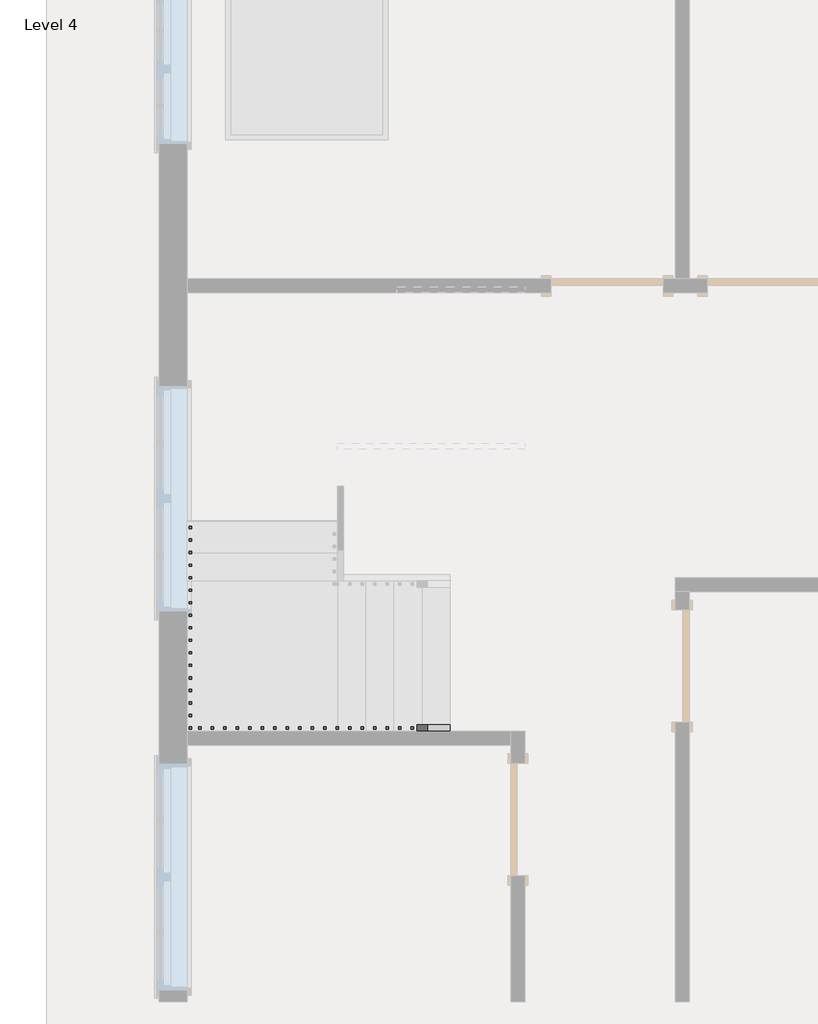
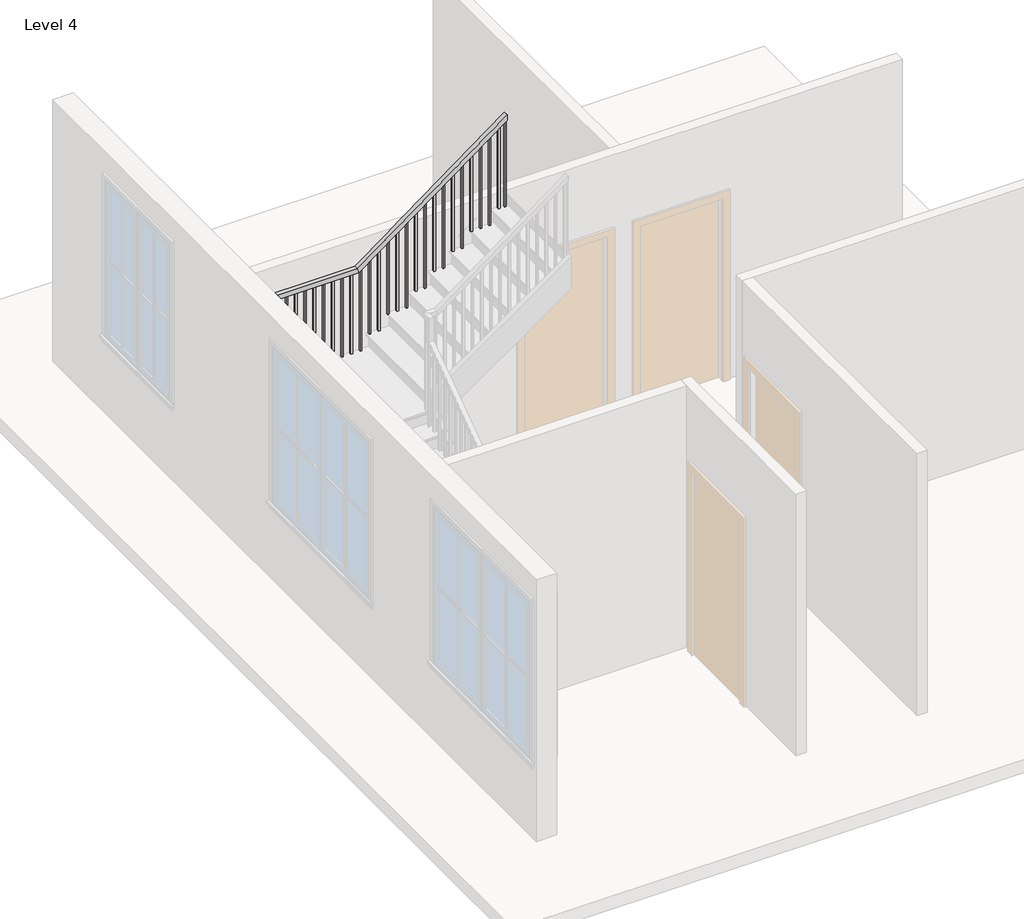
# One storey, part 2 of 3: 1 railing.
"""IFC4 building model written with IfcOpenShell, lengths in millimetres."""

from ifc_helpers import new_model, si_unit, frame, origin, place, context, project, spatial, polyline, outline, extrude, faceted_brep, element, save

model = new_model("IFC4")

# Units and contexts
model_context = context("Model", 3, world=origin())
ifc_project = project(units=[si_unit("LENGTHUNIT", "METRE", prefix="MILLI")], contexts=[model_context])

# Site, building, storey
site = spatial("IfcSite", under=ifc_project)
building = spatial("IfcBuilding", under=site)
storey = spatial("IfcBuildingStorey", under=building, Name="Level 4", Elevation=9448.8)

# Railing
placement = place(None, origin())
element("IfcRailing", 1, ObjectType="Handrail - Rectangular", at=placement, inside=storey, context=model_context, shape_type="SolidModel", body=[
    faceted_brep([(-2683.1105391, -2741.0373761, 10523.6210526), (-2683.1105391, -2741.0373761, 10461.5605986), (-2683.1105391, -2690.2373761, 10461.5605986), (-2683.1105391, -2690.2373761, 10523.6210526), (-3698.24463, -2741.0373761, 11235.9958533), (-3714.290777, -2741.0373761, 11185.1958533), (-3714.290777, -2690.2373761, 11185.1958533), (-3698.24463, -2690.2373761, 11235.9958533), (-4816.7105391, -2741.0373761, 11235.9958533), (-4816.7105391, -2741.0373761, 11185.1958533), (-4765.9105391, -2690.2373761, 11185.1958533), (-4765.9105391, -2690.2373761, 11235.9958533), (-4816.7105391, -1646.8618205, 11235.9958533), (-4816.7105391, -1630.5188912, 11185.1958533), (-4765.9105391, -1630.5188912, 11185.1958533), (-4765.9105391, -1646.8618205, 11235.9958533), (-4816.7105391, -308.3947094, 12196.6181818), (-4816.7105391, -292.0517801, 12145.8181818), (-4765.9105391, -292.0517801, 12145.8181818), (-4765.9105391, -308.3947094, 12196.6181818), (-4816.7105391, 814.9626239, 12196.6181818), (-4816.7105391, 814.9626239, 12145.8181818), (-4765.9105391, 764.1626239, 12145.8181818), (-4765.9105391, 764.1626239, 12196.6181818), (-3721.871578, 814.9626239, 12196.6181818), (-3705.1770744, 814.9626239, 12145.8181818), (-3705.1770744, 764.1626239, 12145.8181818), (-3721.871578, 764.1626239, 12196.6181818), (-2073.5105391, 814.9626239, 13411.2), (-2073.5105391, 764.1626239, 13411.2), (-2073.5105391, 764.1626239, 13348.0987868), (-2073.5105391, 814.9626239, 13348.0987868)], [[[0, 1, 2, 3]], [[1, 0, 4, 5]], [[2, 1, 5, 6]], [[3, 2, 6, 7]], [[0, 3, 7, 4]], [[5, 4, 8, 9]], [[6, 5, 9, 10]], [[7, 6, 10, 11]], [[4, 7, 11, 8]], [[9, 8, 12, 13]], [[10, 9, 13, 14]], [[11, 10, 14, 15]], [[8, 11, 15, 12]], [[13, 12, 16, 17]], [[14, 13, 17, 18]], [[15, 14, 18, 19]], [[12, 15, 19, 16]], [[17, 16, 20, 21]], [[18, 17, 21, 22]], [[19, 18, 22, 23]], [[16, 19, 23, 20]], [[21, 20, 24, 25]], [[22, 21, 25, 26]], [[23, 22, 26, 27]], [[20, 23, 27, 24]], [[28, 29, 30, 31]], [[25, 24, 28, 31]], [[26, 25, 31, 30]], [[27, 26, 30, 29]], [[24, 27, 29, 28]]]),
    extrude(outline(polyline([(13284.9329974, -2159.2355391), (12336.3789474, -2159.2355391), (12336.3789474, -2140.1855391), (13298.9698395, -2140.1855391), (13284.9329974, -2159.2355391)])), frame((0.0, 780.0376239, 0.0), z_axis=(0.0, 1.0, 0.0), x_axis=(0.0, 0.0, 1.0)), (0.0, 0.0, 1.0), 19.05),
    extrude(outline(polyline([(13210.0698395, -2260.8355391), (12175.9578947, -2260.8355391), (12175.9578947, -2241.7855391), (13224.1066816, -2241.7855391), (13210.0698395, -2260.8355391)])), frame((0.0, 780.0376239, 0.0), z_axis=(0.0, 1.0, 0.0), x_axis=(0.0, 0.0, 1.0)), (0.0, 0.0, 1.0), 19.05),
    extrude(outline(polyline([(13135.2066816, -2362.4355391), (12175.9578947, -2362.4355391), (12175.9578947, -2343.3855391), (13149.2435237, -2343.3855391), (13135.2066816, -2362.4355391)])), frame((0.0, 780.0376239, 0.0), z_axis=(0.0, 1.0, 0.0), x_axis=(0.0, 0.0, 1.0)), (0.0, 0.0, 1.0), 19.05),
    extrude(outline(polyline([(13060.3435237, -2464.0355391), (12175.9578947, -2464.0355391), (12175.9578947, -2444.9855391), (13074.3803658, -2444.9855391), (13060.3435237, -2464.0355391)])), frame((0.0, 780.0376239, 0.0), z_axis=(0.0, 1.0, 0.0), x_axis=(0.0, 0.0, 1.0)), (0.0, 0.0, 1.0), 19.05),
    extrude(outline(polyline([(12985.4803658, -2565.6355391), (12015.5368421, -2565.6355391), (12015.5368421, -2546.5855391), (12999.5172079, -2546.5855391), (12985.4803658, -2565.6355391)])), frame((0.0, 780.0376239, 0.0), z_axis=(0.0, 1.0, 0.0), x_axis=(0.0, 0.0, 1.0)), (0.0, 0.0, 1.0), 19.05),
    extrude(outline(polyline([(12910.6172079, -2667.2355391), (12015.5368421, -2667.2355391), (12015.5368421, -2648.1855391), (12924.65405, -2648.1855391), (12910.6172079, -2667.2355391)])), frame((0.0, 780.0376239, 0.0), z_axis=(0.0, 1.0, 0.0), x_axis=(0.0, 0.0, 1.0)), (0.0, 0.0, 1.0), 19.05),
    extrude(outline(polyline([(12835.75405, -2768.8355391), (11855.1157895, -2768.8355391), (11855.1157895, -2749.7855391), (12849.7908921, -2749.7855391), (12835.75405, -2768.8355391)])), frame((0.0, 780.0376239, 0.0), z_axis=(0.0, 1.0, 0.0), x_axis=(0.0, 0.0, 1.0)), (0.0, 0.0, 1.0), 19.05),
    extrude(outline(polyline([(12760.8908921, -2870.4355391), (11855.1157895, -2870.4355391), (11855.1157895, -2851.3855391), (12774.9277342, -2851.3855391), (12760.8908921, -2870.4355391)])), frame((0.0, 780.0376239, 0.0), z_axis=(0.0, 1.0, 0.0), x_axis=(0.0, 0.0, 1.0)), (0.0, 0.0, 1.0), 19.05),
    extrude(outline(polyline([(12686.0277342, -2972.0355391), (11694.6947368, -2972.0355391), (11694.6947368, -2952.9855391), (12700.0645763, -2952.9855391), (12686.0277342, -2972.0355391)])), frame((0.0, 780.0376239, 0.0), z_axis=(0.0, 1.0, 0.0), x_axis=(0.0, 0.0, 1.0)), (0.0, 0.0, 1.0), 19.05),
    extrude(outline(polyline([(12611.1645763, -3073.6355391), (11694.6947368, -3073.6355391), (11694.6947368, -3054.5855391), (12625.2014184, -3054.5855391), (12611.1645763, -3073.6355391)])), frame((0.0, 780.0376239, 0.0), z_axis=(0.0, 1.0, 0.0), x_axis=(0.0, 0.0, 1.0)), (0.0, 0.0, 1.0), 19.05),
    extrude(outline(polyline([(12536.3014184, -3175.2355391), (11534.2736842, -3175.2355391), (11534.2736842, -3156.1855391), (12550.3382605, -3156.1855391), (12536.3014184, -3175.2355391)])), frame((0.0, 780.0376239, 0.0), z_axis=(0.0, 1.0, 0.0), x_axis=(0.0, 0.0, 1.0)), (0.0, 0.0, 1.0), 19.05),
    extrude(outline(polyline([(12461.4382605, -3276.8355391), (11534.2736842, -3276.8355391), (11534.2736842, -3257.7855391), (12475.4751026, -3257.7855391), (12461.4382605, -3276.8355391)])), frame((0.0, 780.0376239, 0.0), z_axis=(0.0, 1.0, 0.0), x_axis=(0.0, 0.0, 1.0)), (0.0, 0.0, 1.0), 19.05),
    extrude(outline(polyline([(12386.5751026, -3378.4355391), (11534.2736842, -3378.4355391), (11534.2736842, -3359.3855391), (12400.6119447, -3359.3855391), (12386.5751026, -3378.4355391)])), frame((0.0, 780.0376239, 0.0), z_axis=(0.0, 1.0, 0.0), x_axis=(0.0, 0.0, 1.0)), (0.0, 0.0, 1.0), 19.05),
    extrude(outline(polyline([(12311.7119447, -3480.0355391), (11373.8526316, -3480.0355391), (11373.8526316, -3460.9855391), (12325.7487868, -3460.9855391), (12311.7119447, -3480.0355391)])), frame((0.0, 780.0376239, 0.0), z_axis=(0.0, 1.0, 0.0), x_axis=(0.0, 0.0, 1.0)), (0.0, 0.0, 1.0), 19.05),
    extrude(outline(polyline([(12236.8487868, -3581.6355391), (11373.8526316, -3581.6355391), (11373.8526316, -3562.5855391), (12250.8856289, -3562.5855391), (12236.8487868, -3581.6355391)])), frame((0.0, 780.0376239, 0.0), z_axis=(0.0, 1.0, 0.0), x_axis=(0.0, 0.0, 1.0)), (0.0, 0.0, 1.0), 19.05),
    extrude(outline(polyline([(12161.9856289, -3683.2355391), (11213.4315789, -3683.2355391), (11213.4315789, -3664.1855391), (12176.022471, -3664.1855391), (12161.9856289, -3683.2355391)])), frame((0.0, 780.0376239, 0.0), z_axis=(0.0, 1.0, 0.0), x_axis=(0.0, 0.0, 1.0)), (0.0, 0.0, 1.0), 19.05),
    extrude(outline(polyline([(-3784.8355391, 799.0876239), (-3765.7855391, 799.0876239), (-3765.7855391, 780.0376239), (-3784.8355391, 780.0376239), (-3784.8355391, 799.0876239)])), frame((0.0, 0.0, 11213.4315789), z_axis=(0.0, 0.0, 1.0), x_axis=(1.0, 0.0, 0.0)), (0.0, 0.0, 1.0), 932.3866029),
    extrude(outline(polyline([(-3886.4355391, 799.0876239), (-3867.3855391, 799.0876239), (-3867.3855391, 780.0376239), (-3886.4355391, 780.0376239), (-3886.4355391, 799.0876239)])), frame((0.0, 0.0, 11213.4315789), z_axis=(0.0, 0.0, 1.0), x_axis=(1.0, 0.0, 0.0)), (0.0, 0.0, 1.0), 932.3866029),
    extrude(outline(polyline([(-3988.0355391, 799.0876239), (-3968.9855391, 799.0876239), (-3968.9855391, 780.0376239), (-3988.0355391, 780.0376239), (-3988.0355391, 799.0876239)])), frame((0.0, 0.0, 11213.4315789), z_axis=(0.0, 0.0, 1.0), x_axis=(1.0, 0.0, 0.0)), (0.0, 0.0, 1.0), 932.3866029),
    extrude(outline(polyline([(-4089.6355391, 799.0876239), (-4070.5855391, 799.0876239), (-4070.5855391, 780.0376239), (-4089.6355391, 780.0376239), (-4089.6355391, 799.0876239)])), frame((0.0, 0.0, 11213.4315789), z_axis=(0.0, 0.0, 1.0), x_axis=(1.0, 0.0, 0.0)), (0.0, 0.0, 1.0), 932.3866029),
    extrude(outline(polyline([(-4191.2355391, 799.0876239), (-4172.1855391, 799.0876239), (-4172.1855391, 780.0376239), (-4191.2355391, 780.0376239), (-4191.2355391, 799.0876239)])), frame((0.0, 0.0, 11213.4315789), z_axis=(0.0, 0.0, 1.0), x_axis=(1.0, 0.0, 0.0)), (0.0, 0.0, 1.0), 932.3866029),
    extrude(outline(polyline([(-4292.8355391, 799.0876239), (-4273.7855391, 799.0876239), (-4273.7855391, 780.0376239), (-4292.8355391, 780.0376239), (-4292.8355391, 799.0876239)])), frame((0.0, 0.0, 11213.4315789), z_axis=(0.0, 0.0, 1.0), x_axis=(1.0, 0.0, 0.0)), (0.0, 0.0, 1.0), 932.3866029),
    extrude(outline(polyline([(-4394.4355391, 799.0876239), (-4375.3855391, 799.0876239), (-4375.3855391, 780.0376239), (-4394.4355391, 780.0376239), (-4394.4355391, 799.0876239)])), frame((0.0, 0.0, 11213.4315789), z_axis=(0.0, 0.0, 1.0), x_axis=(1.0, 0.0, 0.0)), (0.0, 0.0, 1.0), 932.3866029),
    extrude(outline(polyline([(-4496.0355391, 799.0876239), (-4476.9855391, 799.0876239), (-4476.9855391, 780.0376239), (-4496.0355391, 780.0376239), (-4496.0355391, 799.0876239)])), frame((0.0, 0.0, 11213.4315789), z_axis=(0.0, 0.0, 1.0), x_axis=(1.0, 0.0, 0.0)), (0.0, 0.0, 1.0), 932.3866029),
    extrude(outline(polyline([(-4597.6355391, 799.0876239), (-4578.5855391, 799.0876239), (-4578.5855391, 780.0376239), (-4597.6355391, 780.0376239), (-4597.6355391, 799.0876239)])), frame((0.0, 0.0, 11213.4315789), z_axis=(0.0, 0.0, 1.0), x_axis=(1.0, 0.0, 0.0)), (0.0, 0.0, 1.0), 932.3866029),
    extrude(outline(polyline([(-4699.2355391, 799.0876239), (-4680.1855391, 799.0876239), (-4680.1855391, 780.0376239), (-4699.2355391, 780.0376239), (-4699.2355391, 799.0876239)])), frame((0.0, 0.0, 11213.4315789), z_axis=(0.0, 0.0, 1.0), x_axis=(1.0, 0.0, 0.0)), (0.0, 0.0, 1.0), 932.3866029),
    extrude(outline(polyline([(-4800.8355391, 729.2376239), (-4800.8355391, 748.2876239), (-4781.7855391, 748.2876239), (-4781.7855391, 729.2376239), (-4800.8355391, 729.2376239)])), frame((0.0, 0.0, 11213.4315789), z_axis=(0.0, 0.0, 1.0), x_axis=(1.0, 0.0, 0.0)), (0.0, 0.0, 1.0), 932.3866029),
    extrude(outline(polyline([(-4800.8355391, 627.6376239), (-4800.8355391, 646.6876239), (-4781.7855391, 646.6876239), (-4781.7855391, 627.6376239), (-4800.8355391, 627.6376239)])), frame((0.0, 0.0, 11213.4315789), z_axis=(0.0, 0.0, 1.0), x_axis=(1.0, 0.0, 0.0)), (0.0, 0.0, 1.0), 932.3866029),
    extrude(outline(polyline([(-4800.8355391, 526.0376239), (-4800.8355391, 545.0876239), (-4781.7855391, 545.0876239), (-4781.7855391, 526.0376239), (-4800.8355391, 526.0376239)])), frame((0.0, 0.0, 11213.4315789), z_axis=(0.0, 0.0, 1.0), x_axis=(1.0, 0.0, 0.0)), (0.0, 0.0, 1.0), 932.3866029),
    extrude(outline(polyline([(-4800.8355391, 424.4376239), (-4800.8355391, 443.4876239), (-4781.7855391, 443.4876239), (-4781.7855391, 424.4376239), (-4800.8355391, 424.4376239)])), frame((0.0, 0.0, 11213.4315789), z_axis=(0.0, 0.0, 1.0), x_axis=(1.0, 0.0, 0.0)), (0.0, 0.0, 1.0), 932.3866029),
    extrude(outline(polyline([(-4800.8355391, 322.8376239), (-4800.8355391, 341.8876239), (-4781.7855391, 341.8876239), (-4781.7855391, 322.8376239), (-4800.8355391, 322.8376239)])), frame((0.0, 0.0, 11213.4315789), z_axis=(0.0, 0.0, 1.0), x_axis=(1.0, 0.0, 0.0)), (0.0, 0.0, 1.0), 932.3866029),
    extrude(outline(polyline([(-4800.8355391, 221.2376239), (-4800.8355391, 240.2876239), (-4781.7855391, 240.2876239), (-4781.7855391, 221.2376239), (-4800.8355391, 221.2376239)])), frame((0.0, 0.0, 11213.4315789), z_axis=(0.0, 0.0, 1.0), x_axis=(1.0, 0.0, 0.0)), (0.0, 0.0, 1.0), 932.3866029),
    extrude(outline(polyline([(-4800.8355391, 119.6376239), (-4800.8355391, 138.6876239), (-4781.7855391, 138.6876239), (-4781.7855391, 119.6376239), (-4800.8355391, 119.6376239)])), frame((0.0, 0.0, 11213.4315789), z_axis=(0.0, 0.0, 1.0), x_axis=(1.0, 0.0, 0.0)), (0.0, 0.0, 1.0), 932.3866029),
    extrude(outline(polyline([(-4800.8355391, 18.0376239), (-4800.8355391, 37.0876239), (-4781.7855391, 37.0876239), (-4781.7855391, 18.0376239), (-4800.8355391, 18.0376239)])), frame((0.0, 0.0, 11213.4315789), z_axis=(0.0, 0.0, 1.0), x_axis=(1.0, 0.0, 0.0)), (0.0, 0.0, 1.0), 932.3866029),
    extrude(outline(polyline([(-4800.8355391, -83.5623761), (-4800.8355391, -64.5123761), (-4781.7855391, -64.5123761), (-4781.7855391, -83.5623761), (-4800.8355391, -83.5623761)])), frame((0.0, 0.0, 11213.4315789), z_axis=(0.0, 0.0, 1.0), x_axis=(1.0, 0.0, 0.0)), (0.0, 0.0, 1.0), 932.3866029),
    extrude(outline(polyline([(-4800.8355391, -185.1623761), (-4800.8355391, -166.1123761), (-4781.7855391, -166.1123761), (-4781.7855391, -185.1623761), (-4800.8355391, -185.1623761)])), frame((0.0, 0.0, 11213.4315789), z_axis=(0.0, 0.0, 1.0), x_axis=(1.0, 0.0, 0.0)), (0.0, 0.0, 1.0), 932.3866029),
    extrude(outline(polyline([(-4800.8355391, -286.7623761), (-4800.8355391, -267.7123761), (-4781.7855391, -267.7123761), (-4781.7855391, -286.7623761), (-4800.8355391, -286.7623761)])), frame((0.0, 0.0, 11213.4315789), z_axis=(0.0, 0.0, 1.0), x_axis=(1.0, 0.0, 0.0)), (0.0, 0.0, 1.0), 932.3866029),
    extrude(outline(polyline([(-369.3123761, 12090.3679933), (-369.3123761, 11213.4315789), (-388.3623761, 11213.4315789), (-388.3623761, 12076.6957445), (-369.3123761, 12090.3679933)])), frame((-4800.8355391, 0.0, 0.0), z_axis=(1.0, 0.0, 0.0), x_axis=(0.0, 1.0, 0.0)), (0.0, 0.0, 1.0), 19.05),
    extrude(outline(polyline([(-470.9123761, 12017.449333), (-470.9123761, 11053.0105263), (-489.9623761, 11053.0105263), (-489.9623761, 12003.7770842), (-470.9123761, 12017.449333)])), frame((-4800.8355391, 0.0, 0.0), z_axis=(1.0, 0.0, 0.0), x_axis=(0.0, 1.0, 0.0)), (0.0, 0.0, 1.0), 19.05),
    extrude(outline(polyline([(-572.5123761, 11944.5306727), (-572.5123761, 11053.0105263), (-591.5623761, 11053.0105263), (-591.5623761, 11930.8584239), (-572.5123761, 11944.5306727)])), frame((-4800.8355391, 0.0, 0.0), z_axis=(1.0, 0.0, 0.0), x_axis=(0.0, 1.0, 0.0)), (0.0, 0.0, 1.0), 19.05),
    extrude(outline(polyline([(-674.1123761, 11871.6120124), (-674.1123761, 10892.5894737), (-693.1623761, 10892.5894737), (-693.1623761, 11857.9397636), (-674.1123761, 11871.6120124)])), frame((-4800.8355391, 0.0, 0.0), z_axis=(1.0, 0.0, 0.0), x_axis=(0.0, 1.0, 0.0)), (0.0, 0.0, 1.0), 19.05),
    extrude(outline(polyline([(-775.7123761, 11798.6933521), (-775.7123761, 10892.5894737), (-794.7623761, 10892.5894737), (-794.7623761, 11785.0211033), (-775.7123761, 11798.6933521)])), frame((-4800.8355391, 0.0, 0.0), z_axis=(1.0, 0.0, 0.0), x_axis=(0.0, 1.0, 0.0)), (0.0, 0.0, 1.0), 19.05),
    extrude(outline(polyline([(-877.3123761, 11725.7746919), (-877.3123761, 10732.1684211), (-896.3623761, 10732.1684211), (-896.3623761, 11712.102443), (-877.3123761, 11725.7746919)])), frame((-4800.8355391, 0.0, 0.0), z_axis=(1.0, 0.0, 0.0), x_axis=(0.0, 1.0, 0.0)), (0.0, 0.0, 1.0), 19.05),
    extrude(outline(polyline([(-978.9123761, 11652.8560316), (-978.9123761, 10732.1684211), (-997.9623761, 10732.1684211), (-997.9623761, 11639.1837828), (-978.9123761, 11652.8560316)])), frame((-4800.8355391, 0.0, 0.0), z_axis=(1.0, 0.0, 0.0), x_axis=(0.0, 1.0, 0.0)), (0.0, 0.0, 1.0), 19.05),
    extrude(outline(polyline([(-1080.5123761, 11579.9373713), (-1080.5123761, 10571.7473684), (-1099.5623761, 10571.7473684), (-1099.5623761, 11566.2651225), (-1080.5123761, 11579.9373713)])), frame((-4800.8355391, 0.0, 0.0), z_axis=(1.0, 0.0, 0.0), x_axis=(0.0, 1.0, 0.0)), (0.0, 0.0, 1.0), 19.05),
    extrude(outline(polyline([(-1182.1123761, 11507.018711), (-1182.1123761, 10571.7473684), (-1201.1623761, 10571.7473684), (-1201.1623761, 11493.3464622), (-1182.1123761, 11507.018711)])), frame((-4800.8355391, 0.0, 0.0), z_axis=(1.0, 0.0, 0.0), x_axis=(0.0, 1.0, 0.0)), (0.0, 0.0, 1.0), 19.05),
    extrude(outline(polyline([(-1283.7123761, 11434.1000507), (-1283.7123761, 10571.7473684), (-1302.7623761, 10571.7473684), (-1302.7623761, 11420.4278019), (-1283.7123761, 11434.1000507)])), frame((-4800.8355391, 0.0, 0.0), z_axis=(1.0, 0.0, 0.0), x_axis=(0.0, 1.0, 0.0)), (0.0, 0.0, 1.0), 19.05),
    extrude(outline(polyline([(-1385.3123761, 11361.1813904), (-1385.3123761, 10411.3263158), (-1404.3623761, 10411.3263158), (-1404.3623761, 11347.5091416), (-1385.3123761, 11361.1813904)])), frame((-4800.8355391, 0.0, 0.0), z_axis=(1.0, 0.0, 0.0), x_axis=(0.0, 1.0, 0.0)), (0.0, 0.0, 1.0), 19.05),
    extrude(outline(polyline([(-1486.9123761, 11288.2627301), (-1486.9123761, 10411.3263158), (-1505.9623761, 10411.3263158), (-1505.9623761, 11274.5904813), (-1486.9123761, 11288.2627301)])), frame((-4800.8355391, 0.0, 0.0), z_axis=(1.0, 0.0, 0.0), x_axis=(0.0, 1.0, 0.0)), (0.0, 0.0, 1.0), 19.05),
    extrude(outline(polyline([(-1588.5123761, 11215.3440698), (-1588.5123761, 10250.9052632), (-1607.5623761, 10250.9052632), (-1607.5623761, 11201.671821), (-1588.5123761, 11215.3440698)])), frame((-4800.8355391, 0.0, 0.0), z_axis=(1.0, 0.0, 0.0), x_axis=(0.0, 1.0, 0.0)), (0.0, 0.0, 1.0), 19.05),
    extrude(outline(polyline([(-4800.8355391, -1709.1623761), (-4800.8355391, -1690.1123761), (-4781.7855391, -1690.1123761), (-4781.7855391, -1709.1623761), (-4800.8355391, -1709.1623761)])), frame((0.0, 0.0, 10250.9052632), z_axis=(0.0, 0.0, 1.0), x_axis=(1.0, 0.0, 0.0)), (0.0, 0.0, 1.0), 934.2905901),
    extrude(outline(polyline([(-4800.8355391, -1810.7623761), (-4800.8355391, -1791.7123761), (-4781.7855391, -1791.7123761), (-4781.7855391, -1810.7623761), (-4800.8355391, -1810.7623761)])), frame((0.0, 0.0, 10250.9052632), z_axis=(0.0, 0.0, 1.0), x_axis=(1.0, 0.0, 0.0)), (0.0, 0.0, 1.0), 934.2905901),
    extrude(outline(polyline([(-4800.8355391, -1912.3623761), (-4800.8355391, -1893.3123761), (-4781.7855391, -1893.3123761), (-4781.7855391, -1912.3623761), (-4800.8355391, -1912.3623761)])), frame((0.0, 0.0, 10250.9052632), z_axis=(0.0, 0.0, 1.0), x_axis=(1.0, 0.0, 0.0)), (0.0, 0.0, 1.0), 934.2905901),
    extrude(outline(polyline([(-4800.8355391, -2013.9623761), (-4800.8355391, -1994.9123761), (-4781.7855391, -1994.9123761), (-4781.7855391, -2013.9623761), (-4800.8355391, -2013.9623761)])), frame((0.0, 0.0, 10250.9052632), z_axis=(0.0, 0.0, 1.0), x_axis=(1.0, 0.0, 0.0)), (0.0, 0.0, 1.0), 934.2905901),
    extrude(outline(polyline([(-4800.8355391, -2115.5623761), (-4800.8355391, -2096.5123761), (-4781.7855391, -2096.5123761), (-4781.7855391, -2115.5623761), (-4800.8355391, -2115.5623761)])), frame((0.0, 0.0, 10250.9052632), z_axis=(0.0, 0.0, 1.0), x_axis=(1.0, 0.0, 0.0)), (0.0, 0.0, 1.0), 934.2905901),
    extrude(outline(polyline([(-4800.8355391, -2217.1623761), (-4800.8355391, -2198.1123761), (-4781.7855391, -2198.1123761), (-4781.7855391, -2217.1623761), (-4800.8355391, -2217.1623761)])), frame((0.0, 0.0, 10250.9052632), z_axis=(0.0, 0.0, 1.0), x_axis=(1.0, 0.0, 0.0)), (0.0, 0.0, 1.0), 934.2905901),
    extrude(outline(polyline([(-4800.8355391, -2318.7623761), (-4800.8355391, -2299.7123761), (-4781.7855391, -2299.7123761), (-4781.7855391, -2318.7623761), (-4800.8355391, -2318.7623761)])), frame((0.0, 0.0, 10250.9052632), z_axis=(0.0, 0.0, 1.0), x_axis=(1.0, 0.0, 0.0)), (0.0, 0.0, 1.0), 934.2905901),
    extrude(outline(polyline([(-4800.8355391, -2420.3623761), (-4800.8355391, -2401.3123761), (-4781.7855391, -2401.3123761), (-4781.7855391, -2420.3623761), (-4800.8355391, -2420.3623761)])), frame((0.0, 0.0, 10250.9052632), z_axis=(0.0, 0.0, 1.0), x_axis=(1.0, 0.0, 0.0)), (0.0, 0.0, 1.0), 934.2905901),
    extrude(outline(polyline([(-4800.8355391, -2521.9623761), (-4800.8355391, -2502.9123761), (-4781.7855391, -2502.9123761), (-4781.7855391, -2521.9623761), (-4800.8355391, -2521.9623761)])), frame((0.0, 0.0, 10250.9052632), z_axis=(0.0, 0.0, 1.0), x_axis=(1.0, 0.0, 0.0)), (0.0, 0.0, 1.0), 934.2905901),
    extrude(outline(polyline([(-4800.8355391, -2623.5623761), (-4800.8355391, -2604.5123761), (-4781.7855391, -2604.5123761), (-4781.7855391, -2623.5623761), (-4800.8355391, -2623.5623761)])), frame((0.0, 0.0, 10250.9052632), z_axis=(0.0, 0.0, 1.0), x_axis=(1.0, 0.0, 0.0)), (0.0, 0.0, 1.0), 934.2905901),
    extrude(outline(polyline([(-4705.5855391, -2725.1623761), (-4724.6355391, -2725.1623761), (-4724.6355391, -2706.1123761), (-4705.5855391, -2706.1123761), (-4705.5855391, -2725.1623761)])), frame((0.0, 0.0, 10250.9052632), z_axis=(0.0, 0.0, 1.0), x_axis=(1.0, 0.0, 0.0)), (0.0, 0.0, 1.0), 934.2905901),
    extrude(outline(polyline([(-4603.9855391, -2725.1623761), (-4623.0355391, -2725.1623761), (-4623.0355391, -2706.1123761), (-4603.9855391, -2706.1123761), (-4603.9855391, -2725.1623761)])), frame((0.0, 0.0, 10250.9052632), z_axis=(0.0, 0.0, 1.0), x_axis=(1.0, 0.0, 0.0)), (0.0, 0.0, 1.0), 934.2905901),
    extrude(outline(polyline([(-4502.3855391, -2725.1623761), (-4521.4355391, -2725.1623761), (-4521.4355391, -2706.1123761), (-4502.3855391, -2706.1123761), (-4502.3855391, -2725.1623761)])), frame((0.0, 0.0, 10250.9052632), z_axis=(0.0, 0.0, 1.0), x_axis=(1.0, 0.0, 0.0)), (0.0, 0.0, 1.0), 934.2905901),
    extrude(outline(polyline([(-4400.7855391, -2725.1623761), (-4419.8355391, -2725.1623761), (-4419.8355391, -2706.1123761), (-4400.7855391, -2706.1123761), (-4400.7855391, -2725.1623761)])), frame((0.0, 0.0, 10250.9052632), z_axis=(0.0, 0.0, 1.0), x_axis=(1.0, 0.0, 0.0)), (0.0, 0.0, 1.0), 934.2905901),
    extrude(outline(polyline([(-4299.1855391, -2725.1623761), (-4318.2355391, -2725.1623761), (-4318.2355391, -2706.1123761), (-4299.1855391, -2706.1123761), (-4299.1855391, -2725.1623761)])), frame((0.0, 0.0, 10250.9052632), z_axis=(0.0, 0.0, 1.0), x_axis=(1.0, 0.0, 0.0)), (0.0, 0.0, 1.0), 934.2905901),
    extrude(outline(polyline([(-4197.5855391, -2725.1623761), (-4216.6355391, -2725.1623761), (-4216.6355391, -2706.1123761), (-4197.5855391, -2706.1123761), (-4197.5855391, -2725.1623761)])), frame((0.0, 0.0, 10250.9052632), z_axis=(0.0, 0.0, 1.0), x_axis=(1.0, 0.0, 0.0)), (0.0, 0.0, 1.0), 934.2905901),
    extrude(outline(polyline([(-4095.9855391, -2725.1623761), (-4115.0355391, -2725.1623761), (-4115.0355391, -2706.1123761), (-4095.9855391, -2706.1123761), (-4095.9855391, -2725.1623761)])), frame((0.0, 0.0, 10250.9052632), z_axis=(0.0, 0.0, 1.0), x_axis=(1.0, 0.0, 0.0)), (0.0, 0.0, 1.0), 934.2905901),
    extrude(outline(polyline([(-3994.3855391, -2725.1623761), (-4013.4355391, -2725.1623761), (-4013.4355391, -2706.1123761), (-3994.3855391, -2706.1123761), (-3994.3855391, -2725.1623761)])), frame((0.0, 0.0, 10250.9052632), z_axis=(0.0, 0.0, 1.0), x_axis=(1.0, 0.0, 0.0)), (0.0, 0.0, 1.0), 934.2905901),
    extrude(outline(polyline([(-3892.7855391, -2725.1623761), (-3911.8355391, -2725.1623761), (-3911.8355391, -2706.1123761), (-3892.7855391, -2706.1123761), (-3892.7855391, -2725.1623761)])), frame((0.0, 0.0, 10250.9052632), z_axis=(0.0, 0.0, 1.0), x_axis=(1.0, 0.0, 0.0)), (0.0, 0.0, 1.0), 934.2905901),
    extrude(outline(polyline([(-3791.1855391, -2725.1623761), (-3810.2355391, -2725.1623761), (-3810.2355391, -2706.1123761), (-3791.1855391, -2706.1123761), (-3791.1855391, -2725.1623761)])), frame((0.0, 0.0, 10250.9052632), z_axis=(0.0, 0.0, 1.0), x_axis=(1.0, 0.0, 0.0)), (0.0, 0.0, 1.0), 934.2905901),
    extrude(outline(polyline([(-3689.5855391, -2725.1623761), (-3708.6355391, -2725.1623761), (-3708.6355391, -2706.1123761), (-3689.5855391, -2706.1123761), (-3689.5855391, -2725.1623761)])), frame((0.0, 0.0, 10250.9052632), z_axis=(0.0, 0.0, 1.0), x_axis=(1.0, 0.0, 0.0)), (0.0, 0.0, 1.0), 934.2905901),
    extrude(outline(polyline([(11109.9290196, -3607.0355391), (10250.9052632, -3607.0355391), (10250.9052632, -3587.9855391), (11096.5605986, -3587.9855391), (11109.9290196, -3607.0355391)])), frame((0.0, -2725.1623761, 0.0), z_axis=(0.0, 1.0, 0.0), x_axis=(0.0, 0.0, 1.0)), (0.0, 0.0, 1.0), 19.05),
    extrude(outline(polyline([(11038.630774, -3505.4355391), (10090.4842105, -3505.4355391), (10090.4842105, -3486.3855391), (11025.262353, -3486.3855391), (11038.630774, -3505.4355391)])), frame((0.0, -2725.1623761, 0.0), z_axis=(0.0, 1.0, 0.0), x_axis=(0.0, 0.0, 1.0)), (0.0, 0.0, 1.0), 19.05),
    extrude(outline(polyline([(10967.3325284, -3403.8355391), (10090.4842105, -3403.8355391), (10090.4842105, -3384.7855391), (10953.9641074, -3384.7855391), (10967.3325284, -3403.8355391)])), frame((0.0, -2725.1623761, 0.0), z_axis=(0.0, 1.0, 0.0), x_axis=(0.0, 0.0, 1.0)), (0.0, 0.0, 1.0), 19.05),
    extrude(outline(polyline([(10896.0342828, -3302.2355391), (9930.0631579, -3302.2355391), (9930.0631579, -3283.1855391), (10882.6658617, -3283.1855391), (10896.0342828, -3302.2355391)])), frame((0.0, -2725.1623761, 0.0), z_axis=(0.0, 1.0, 0.0), x_axis=(0.0, 0.0, 1.0)), (0.0, 0.0, 1.0), 19.05),
    extrude(outline(polyline([(10824.7360372, -3200.6355391), (9930.0631579, -3200.6355391), (9930.0631579, -3181.5855391), (10811.3676161, -3181.5855391), (10824.7360372, -3200.6355391)])), frame((0.0, -2725.1623761, 0.0), z_axis=(0.0, 1.0, 0.0), x_axis=(0.0, 0.0, 1.0)), (0.0, 0.0, 1.0), 19.05),
    extrude(outline(polyline([(10753.4377916, -3099.0355391), (9769.6421053, -3099.0355391), (9769.6421053, -3079.9855391), (10740.0693705, -3079.9855391), (10753.4377916, -3099.0355391)])), frame((0.0, -2725.1623761, 0.0), z_axis=(0.0, 1.0, 0.0), x_axis=(0.0, 0.0, 1.0)), (0.0, 0.0, 1.0), 19.05),
    extrude(outline(polyline([(10682.1395459, -2997.4355391), (9769.6421053, -2997.4355391), (9769.6421053, -2978.3855391), (10668.7711249, -2978.3855391), (10682.1395459, -2997.4355391)])), frame((0.0, -2725.1623761, 0.0), z_axis=(0.0, 1.0, 0.0), x_axis=(0.0, 0.0, 1.0)), (0.0, 0.0, 1.0), 19.05),
    extrude(outline(polyline([(10610.8413003, -2895.8355391), (9609.2210526, -2895.8355391), (9609.2210526, -2876.7855391), (10597.4728793, -2876.7855391), (10610.8413003, -2895.8355391)])), frame((0.0, -2725.1623761, 0.0), z_axis=(0.0, 1.0, 0.0), x_axis=(0.0, 0.0, 1.0)), (0.0, 0.0, 1.0), 19.05),
    extrude(outline(polyline([(10539.5430547, -2794.2355391), (9609.2210526, -2794.2355391), (9609.2210526, -2775.1855391), (10526.1746337, -2775.1855391), (10539.5430547, -2794.2355391)])), frame((0.0, -2725.1623761, 0.0), z_axis=(0.0, 1.0, 0.0), x_axis=(0.0, 0.0, 1.0)), (0.0, 0.0, 1.0), 19.05),
    extrude(outline(polyline([(-4800.8355391, 780.0376239), (-4800.8355391, 799.0876239), (-4781.7855391, 799.0876239), (-4781.7855391, 780.0376239), (-4800.8355391, 780.0376239)])), frame((0.0, 0.0, 11213.4315789), z_axis=(0.0, 0.0, 1.0), x_axis=(1.0, 0.0, 0.0)), (0.0, 0.0, 1.0), 932.3866029),
    extrude(outline(polyline([(-4781.7855391, -2725.1623761), (-4800.8355391, -2725.1623761), (-4800.8355391, -2706.1123761), (-4781.7855391, -2706.1123761), (-4781.7855391, -2725.1623761)])), frame((0.0, 0.0, 10250.9052632), z_axis=(0.0, 0.0, 1.0), x_axis=(1.0, 0.0, 0.0)), (0.0, 0.0, 1.0), 934.2905901),
    extrude(outline(polyline([(13334.0619447, -2092.5605391), (12336.3789474, -2092.5605391), (12336.3789474, -2073.5105391), (13348.0987868, -2073.5105391), (13334.0619447, -2092.5605391)])), frame((0.0, 780.0376239, 0.0), z_axis=(0.0, 1.0, 0.0), x_axis=(0.0, 0.0, 1.0)), (0.0, 0.0, 1.0), 19.05),
    extrude(outline(polyline([(10474.9290196, -2702.1605391), (9609.2210526, -2702.1605391), (9609.2210526, -2683.1105391), (10461.5605986, -2683.1105391), (10474.9290196, -2702.1605391)])), frame((0.0, -2725.1623761, 0.0), z_axis=(0.0, 1.0, 0.0), x_axis=(0.0, 0.0, 1.0)), (0.0, 0.0, 1.0), 19.05),
])

save(model, "model.ifc")

# Revit data of these elements
# Type "Handrail - Rectangular"
#   Assembly Code = "C2010400"
#   built-in parameter 1008612 = 0.0416667 (stored number, unit not read)
#   built-in parameter 1008611 = 0.0416667 (stored number, unit not read)
#   built-in parameter 1008609 = 0.333333 (stored number, unit not read)
#   built-in parameter 1008604 = 0.166667 (stored number, unit not read)
#   built-in parameter 1008603 = 0.166667 (stored number, unit not read)
#   Railing Height = 3' - 0"
#   built-in parameter 1008630 = 2
#   built-in parameter 1008610 = 2
#   built-in parameter 1008618 = Baluster - Square : 3/4"
# Element 1 (IfcRailing, "Handrail - Rectangular")
#   Phase Created = New Construction
